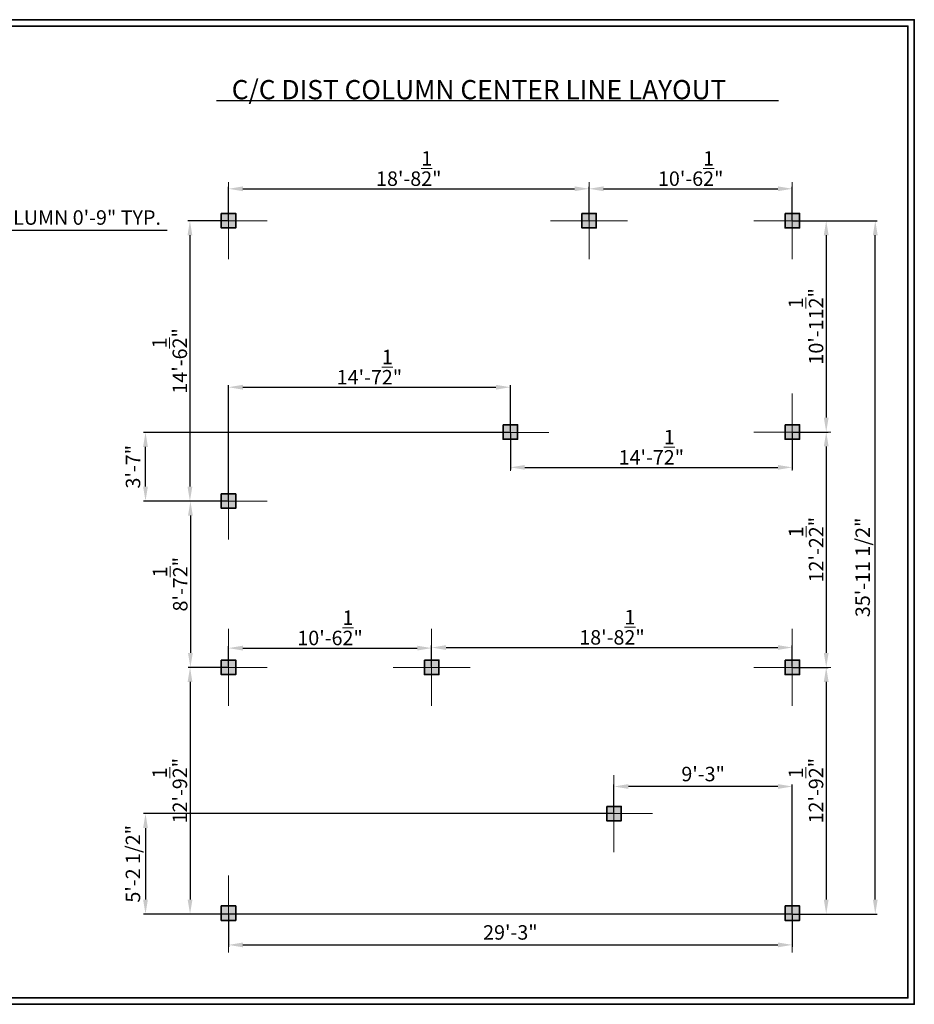
# Model space of a CAD drawing. Units: inches. Extents: x 2436 to 3928, y 1526 to 2149.
# Tile 6 of 6: x 3371 to 3928, y 1526 to 2138. Entities that reach past the tile are written whole.
import ezdxf

# ---------------------------------------------------------------- set-up
doc = ezdxf.new("R2010")
doc.units = ezdxf.units.IN
for name, color, linetype, lineweight in [('G-ANNO-TEXT', 7, 'Continuous', 25), ('G-ANNO-TTLB', 7, 'Continuous', 35), ('S-ANNO-DIMS', 2, 'Continuous', 18), ('S-COLS', 1, 'Continuous', 35), ('S-COLS-MARK', 7, 'Continuous', 13), ('S-COLS-PATT', 1, 'Continuous', 13)]:
    doc.layers.add(name, color=color, linetype=linetype, lineweight=lineweight)
doc.styles.get("Standard").update_dxf_attribs({"font": 'arial.ttf'})
doc.dimstyles.new('ISO-25', dxfattribs={"dimtxt": 9, "dimasz": 9, "dimexe": 1.25, "dimexo": 0.625, "dimgap": 2, "dimtad": 1, "dimdec": 1, "dimlunit": 4, "dimtxsty": 'Standard', "dimcen": 2.5, "dimadec": 0, "dimazin": 0, "dimtfac": 1, "dimtdec": 1, "dimtmove": 0, "dimatfit": 3, "dimfxl": 1, "dimarcsym": 0})

# ---------------------------------------------------------------- blocks, each defined once
blk = doc.blocks.new('*D10')
at = {"layer": 'Defpoints', "color": 0, "transparency": 16777216}
for p in [(3500.55, 2013.29), (3476.55, 1838.79), (3500.55, 1838.79)]:
    blk.add_point(p, dxfattribs=at)
at = {"layer": 'S-ANNO-DIMS', "color": 0, "lineweight": -2, "transparency": 16777216}
for p, q in [((3499.93, 2013.29), (3475.3, 2013.29)), ((3476.55, 2004.29), (3476.55, 1847.79)), ((3499.93, 1838.79), (3475.3, 1838.79))]:
    blk.add_line(p, q, dxfattribs=at)
at = {"layer": 'S-ANNO-DIMS', "color": 0, "transparency": 16777216}
for points in [[(3475.05, 2004.29), (3478.05, 2004.29), (3476.55, 2013.29)], [(3475.05, 1847.79), (3478.05, 1847.79), (3476.55, 1838.79)]]:
    blk.add_solid(points, dxfattribs=at)
at = {"layer": 'S-ANNO-DIMS', "color": 0, "transparency": 16777216, "insert": (3463.94, 1926.04), "char_height": 9, "attachment_point": 5, "rotation": 90}
blk.add_mtext('14\'-6{\\H1x;\\S1/2;}"', dxfattribs=at)
blk = doc.blocks.new('*D11')
at = {"layer": 'Defpoints', "color": 0, "transparency": 16777216}
for p in [(3500.55, 1838.79), (3476.86, 1735.29), (3500.55, 1735.29)]:
    blk.add_point(p, dxfattribs=at)
at = {"layer": 'S-ANNO-DIMS', "color": 0, "lineweight": -2, "transparency": 16777216}
for p, q in [((3499.93, 1838.79), (3475.61, 1838.79)), ((3476.86, 1829.79), (3476.86, 1744.29)), ((3499.93, 1735.29), (3475.61, 1735.29))]:
    blk.add_line(p, q, dxfattribs=at)
at = {"layer": 'S-ANNO-DIMS', "color": 0, "transparency": 16777216}
for points in [[(3475.36, 1829.79), (3478.36, 1829.79), (3476.86, 1838.79)], [(3475.36, 1744.29), (3478.36, 1744.29), (3476.86, 1735.29)]]:
    blk.add_solid(points, dxfattribs=at)
at = {"layer": 'S-ANNO-DIMS', "color": 0, "transparency": 16777216, "insert": (3464.24, 1787.04), "char_height": 9, "attachment_point": 5, "rotation": 90}
blk.add_mtext('8\'-7{\\H1x;\\S1/2;}"', dxfattribs=at)
blk = doc.blocks.new('*D12')
at = {"layer": 'Defpoints', "color": 0, "transparency": 16777216}
for p in [(3500.55, 1735.29), (3476.63, 1581.79), (3500.55, 1581.79)]:
    blk.add_point(p, dxfattribs=at)
at = {"layer": 'S-ANNO-DIMS', "color": 0, "lineweight": -2, "transparency": 16777216}
for p, q in [((3499.93, 1735.29), (3475.38, 1735.29)), ((3476.63, 1726.29), (3476.63, 1590.79)), ((3499.93, 1581.79), (3475.38, 1581.79))]:
    blk.add_line(p, q, dxfattribs=at)
at = {"layer": 'S-ANNO-DIMS', "color": 0, "transparency": 16777216}
for points in [[(3475.13, 1726.29), (3478.13, 1726.29), (3476.63, 1735.29)], [(3475.13, 1590.79), (3478.13, 1590.79), (3476.63, 1581.79)]]:
    blk.add_solid(points, dxfattribs=at)
at = {"layer": 'S-ANNO-DIMS', "color": 0, "transparency": 16777216, "insert": (3464.01, 1658.54), "char_height": 9, "attachment_point": 5, "rotation": 90}
blk.add_mtext('12\'-9{\\H1x;\\S1/2;}"', dxfattribs=at)
blk = doc.blocks.new('*D13')
at = {"layer": 'Defpoints', "color": 0, "transparency": 16777216}
for p in [(3500.55, 1581.79), (3851.55, 1581.79), (3851.55, 1562.57)]:
    blk.add_point(p, dxfattribs=at)
at = {"layer": 'S-ANNO-DIMS', "color": 0, "lineweight": -2, "transparency": 16777216}
for p, q in [((3500.55, 1581.16), (3500.55, 1561.32)), ((3851.55, 1581.16), (3851.55, 1561.32)), ((3509.55, 1562.57), (3842.55, 1562.57))]:
    blk.add_line(p, q, dxfattribs=at)
at = {"layer": 'S-ANNO-DIMS', "color": 0, "transparency": 16777216}
for points in [[(3509.55, 1564.07), (3509.55, 1561.07), (3500.55, 1562.57)], [(3842.55, 1564.07), (3842.55, 1561.07), (3851.55, 1562.57)]]:
    blk.add_solid(points, dxfattribs=at)
at = {"layer": 'S-ANNO-DIMS', "color": 0, "transparency": 16777216, "insert": (3676.05, 1569.17), "char_height": 9, "attachment_point": 5}
blk.add_mtext('29\'-3"', dxfattribs=at)
blk = doc.blocks.new('*D14')
at = {"layer": 'Defpoints', "color": 0, "transparency": 16777216}
for p in [(3851.55, 1735.29), (3851.55, 1581.79), (3872.67, 1581.79)]:
    blk.add_point(p, dxfattribs=at)
at = {"layer": 'S-ANNO-DIMS', "color": 0, "lineweight": -2, "transparency": 16777216}
for p, q in [((3852.18, 1735.29), (3873.92, 1735.29)), ((3872.67, 1726.29), (3872.67, 1590.79)), ((3852.18, 1581.79), (3873.92, 1581.79))]:
    blk.add_line(p, q, dxfattribs=at)
at = {"layer": 'S-ANNO-DIMS', "color": 0, "transparency": 16777216}
for points in [[(3871.17, 1726.29), (3874.17, 1726.29), (3872.67, 1735.29)], [(3871.17, 1590.79), (3874.17, 1590.79), (3872.67, 1581.79)]]:
    blk.add_solid(points, dxfattribs=at)
at = {"layer": 'S-ANNO-DIMS', "color": 0, "transparency": 16777216, "insert": (3860.05, 1658.54), "char_height": 9, "attachment_point": 5, "rotation": 90}
blk.add_mtext('12\'-9{\\H1x;\\S1/2;}"', dxfattribs=at)
blk = doc.blocks.new('*D15')
at = {"layer": 'Defpoints', "color": 0, "transparency": 16777216}
for p in [(3851.55, 1881.79), (3851.55, 1735.29), (3872.67, 1735.29)]:
    blk.add_point(p, dxfattribs=at)
at = {"layer": 'S-ANNO-DIMS', "color": 0, "lineweight": -2, "transparency": 16777216}
for p, q in [((3852.18, 1881.79), (3873.92, 1881.79)), ((3872.67, 1872.79), (3872.67, 1744.29)), ((3852.18, 1735.29), (3873.92, 1735.29))]:
    blk.add_line(p, q, dxfattribs=at)
at = {"layer": 'S-ANNO-DIMS', "color": 0, "transparency": 16777216}
for points in [[(3871.17, 1872.79), (3874.17, 1872.79), (3872.67, 1881.79)], [(3871.17, 1744.29), (3874.17, 1744.29), (3872.67, 1735.29)]]:
    blk.add_solid(points, dxfattribs=at)
at = {"layer": 'S-ANNO-DIMS', "color": 0, "transparency": 16777216, "insert": (3860.13, 1808.54), "char_height": 9, "attachment_point": 5, "rotation": 90}
blk.add_mtext('12\'-2{\\H1x;\\S1/2;}"', dxfattribs=at)
blk = doc.blocks.new('*D16')
at = {"layer": 'Defpoints', "color": 0, "transparency": 16777216}
for p in [(3851.55, 2013.29), (3851.55, 1881.79), (3872.67, 1881.79)]:
    blk.add_point(p, dxfattribs=at)
at = {"layer": 'S-ANNO-DIMS', "color": 0, "lineweight": -2, "transparency": 16777216}
for p, q in [((3852.18, 2013.29), (3873.92, 2013.29)), ((3872.67, 2004.29), (3872.67, 1890.79)), ((3852.18, 1881.79), (3873.92, 1881.79))]:
    blk.add_line(p, q, dxfattribs=at)
at = {"layer": 'S-ANNO-DIMS', "color": 0, "transparency": 16777216}
for points in [[(3871.17, 2004.29), (3874.17, 2004.29), (3872.67, 2013.29)], [(3871.17, 1890.79), (3874.17, 1890.79), (3872.67, 1881.79)]]:
    blk.add_solid(points, dxfattribs=at)
at = {"layer": 'S-ANNO-DIMS', "color": 0, "transparency": 16777216, "insert": (3860.05, 1947.54), "char_height": 9, "attachment_point": 5, "rotation": 90}
blk.add_mtext('10\'-11{\\H1x;\\S1/2;}"', dxfattribs=at)
blk = doc.blocks.new('*D17')
at = {"layer": 'Defpoints', "color": 0, "transparency": 16777216}
for p in [(3851.55, 2033.16), (3725.05, 2013.29), (3851.55, 2013.29)]:
    blk.add_point(p, dxfattribs=at)
at = {"layer": 'S-ANNO-DIMS', "color": 0, "lineweight": -2, "transparency": 16777216}
for p, q in [((3725.05, 2013.91), (3725.05, 2034.41)), ((3734.05, 2033.16), (3842.55, 2033.16)), ((3851.55, 2013.91), (3851.55, 2034.41))]:
    blk.add_line(p, q, dxfattribs=at)
at = {"layer": 'S-ANNO-DIMS', "color": 0, "transparency": 16777216}
for points in [[(3734.05, 2034.66), (3734.05, 2031.66), (3725.05, 2033.16)], [(3842.55, 2034.66), (3842.55, 2031.66), (3851.55, 2033.16)]]:
    blk.add_solid(points, dxfattribs=at)
at = {"layer": 'S-ANNO-DIMS', "color": 0, "transparency": 16777216, "insert": (3788.3, 2045.77), "char_height": 9, "attachment_point": 5}
blk.add_mtext('10\'-6{\\H1x;\\S1/2;}"', dxfattribs=at)
blk = doc.blocks.new('*D18')
at = {"layer": 'Defpoints', "color": 0, "transparency": 16777216}
for p in [(3725.05, 2033.16), (3500.55, 2013.29), (3725.05, 2013.29)]:
    blk.add_point(p, dxfattribs=at)
at = {"layer": 'S-ANNO-DIMS', "color": 0, "lineweight": -2, "transparency": 16777216}
for p, q in [((3500.55, 2013.91), (3500.55, 2034.41)), ((3509.55, 2033.16), (3716.05, 2033.16)), ((3725.05, 2013.91), (3725.05, 2034.41))]:
    blk.add_line(p, q, dxfattribs=at)
at = {"layer": 'S-ANNO-DIMS', "color": 0, "transparency": 16777216}
for points in [[(3509.55, 2034.66), (3509.55, 2031.66), (3500.55, 2033.16)], [(3716.05, 2034.66), (3716.05, 2031.66), (3725.05, 2033.16)]]:
    blk.add_solid(points, dxfattribs=at)
at = {"layer": 'S-ANNO-DIMS', "color": 0, "transparency": 16777216, "insert": (3612.8, 2045.77), "char_height": 9, "attachment_point": 5}
blk.add_mtext('18\'-8{\\H1x;\\S1/2;}"', dxfattribs=at)
blk = doc.blocks.new('*D19')
at = {"layer": 'Defpoints', "color": 0, "transparency": 16777216}
for p in [(3627.05, 1747.29), (3500.55, 1735.29), (3627.05, 1735.29)]:
    blk.add_point(p, dxfattribs=at)
at = {"layer": 'S-ANNO-DIMS', "color": 0, "lineweight": -2, "transparency": 16777216}
for p, q in [((3500.55, 1735.91), (3500.55, 1748.54)), ((3509.55, 1747.29), (3618.05, 1747.29)), ((3627.05, 1735.91), (3627.05, 1748.54))]:
    blk.add_line(p, q, dxfattribs=at)
at = {"layer": 'S-ANNO-DIMS', "color": 0, "transparency": 16777216}
for points in [[(3509.55, 1748.79), (3509.55, 1745.79), (3500.55, 1747.29)], [(3618.05, 1748.79), (3618.05, 1745.79), (3627.05, 1747.29)]]:
    blk.add_solid(points, dxfattribs=at)
at = {"layer": 'S-ANNO-DIMS', "color": 0, "transparency": 16777216, "insert": (3563.8, 1759.9), "char_height": 9, "attachment_point": 5}
blk.add_mtext('10\'-6{\\H1x;\\S1/2;}"', dxfattribs=at)
blk = doc.blocks.new('*D20')
at = {"layer": 'Defpoints', "color": 0, "transparency": 16777216}
for p in [(3851.55, 1747.65), (3627.05, 1735.29), (3851.55, 1735.29)]:
    blk.add_point(p, dxfattribs=at)
at = {"layer": 'S-ANNO-DIMS', "color": 0, "lineweight": -2, "transparency": 16777216}
for p, q in [((3627.05, 1735.91), (3627.05, 1748.9)), ((3636.05, 1747.65), (3842.55, 1747.65)), ((3851.55, 1735.91), (3851.55, 1748.9))]:
    blk.add_line(p, q, dxfattribs=at)
at = {"layer": 'S-ANNO-DIMS', "color": 0, "transparency": 16777216}
for points in [[(3636.05, 1749.15), (3636.05, 1746.15), (3627.05, 1747.65)], [(3842.55, 1749.15), (3842.55, 1746.15), (3851.55, 1747.65)]]:
    blk.add_solid(points, dxfattribs=at)
at = {"layer": 'S-ANNO-DIMS', "color": 0, "transparency": 16777216, "insert": (3739.3, 1760.27), "char_height": 9, "attachment_point": 5}
blk.add_mtext('18\'-8{\\H1x;\\S1/2;}"', dxfattribs=at)
blk = doc.blocks.new('*D21')
at = {"layer": 'Defpoints', "color": 0, "transparency": 16777216}
for p in [(3676.05, 1881.55), (3851.55, 1881.79), (3851.55, 1859.78)]:
    blk.add_point(p, dxfattribs=at)
at = {"layer": 'S-ANNO-DIMS', "color": 0, "lineweight": -2, "transparency": 16777216}
for p, q in [((3676.05, 1880.93), (3676.05, 1858.53)), ((3851.55, 1881.16), (3851.55, 1858.53)), ((3685.05, 1859.78), (3842.55, 1859.78))]:
    blk.add_line(p, q, dxfattribs=at)
at = {"layer": 'S-ANNO-DIMS', "color": 0, "transparency": 16777216}
for points in [[(3685.05, 1861.28), (3685.05, 1858.28), (3676.05, 1859.78)], [(3842.55, 1861.28), (3842.55, 1858.28), (3851.55, 1859.78)]]:
    blk.add_solid(points, dxfattribs=at)
at = {"layer": 'S-ANNO-DIMS', "color": 0, "transparency": 16777216, "insert": (3763.8, 1872.32), "char_height": 9, "attachment_point": 5}
blk.add_mtext('14\'-7{\\H1x;\\S1/2;}"', dxfattribs=at)
blk = doc.blocks.new('*D22')
at = {"layer": 'Defpoints', "color": 0, "transparency": 16777216}
for p in [(3676.05, 1909.66), (3676.05, 1881.55), (3500.55, 1838.79)]:
    blk.add_point(p, dxfattribs=at)
at = {"layer": 'S-ANNO-DIMS', "color": 0, "lineweight": -2, "transparency": 16777216}
for p, q in [((3500.55, 1839.41), (3500.55, 1910.91)), ((3509.55, 1909.66), (3667.05, 1909.66)), ((3676.05, 1882.18), (3676.05, 1910.91))]:
    blk.add_line(p, q, dxfattribs=at)
at = {"layer": 'S-ANNO-DIMS', "color": 0, "transparency": 16777216}
for points in [[(3509.55, 1911.16), (3509.55, 1908.16), (3500.55, 1909.66)], [(3667.05, 1911.16), (3667.05, 1908.16), (3676.05, 1909.66)]]:
    blk.add_solid(points, dxfattribs=at)
at = {"layer": 'S-ANNO-DIMS', "color": 0, "transparency": 16777216, "insert": (3588.3, 1922.19), "char_height": 9, "attachment_point": 5}
blk.add_mtext('14\'-7{\\H1x;\\S1/2;}"', dxfattribs=at)
blk = doc.blocks.new('*D23')
at = {"layer": 'Defpoints', "color": 0, "transparency": 16777216}
for p in [(3740.55, 1661.15), (3740.55, 1644.29), (3851.55, 1581.79)]:
    blk.add_point(p, dxfattribs=at)
at = {"layer": 'S-ANNO-DIMS', "color": 0, "lineweight": -2, "transparency": 16777216}
for p, q in [((3740.55, 1644.91), (3740.55, 1662.4)), ((3842.55, 1661.15), (3749.55, 1661.15)), ((3851.55, 1582.41), (3851.55, 1662.4))]:
    blk.add_line(p, q, dxfattribs=at)
at = {"layer": 'S-ANNO-DIMS', "color": 0, "transparency": 16777216}
for points in [[(3749.55, 1662.65), (3749.55, 1659.65), (3740.55, 1661.15)], [(3842.55, 1662.65), (3842.55, 1659.65), (3851.55, 1661.15)]]:
    blk.add_solid(points, dxfattribs=at)
at = {"layer": 'S-ANNO-DIMS', "color": 0, "transparency": 16777216, "insert": (3796.05, 1667.74), "char_height": 9, "attachment_point": 5}
blk.add_mtext('9\'-3"', dxfattribs=at)
blk = doc.blocks.new('COL-9x9-PLAN')
h = blk.add_hatch(color=256)
h.dxf.hatch_style = 1
h.paths.add_polyline_path([(9, 0), (9, 9), (0, 9), (0, 0)])
blk.add_lwpolyline([(0, 9), (9, 9), (9, 0), (0, 0)], close=True)
blk = doc.blocks.new('COLUMN-CENTER-MARK')
for q in [(24, 48), (0, 24), (48, 24), (24, 0)]:
    blk.add_line((24, 24), q)
blk = doc.blocks.new('*D30')
at = {"layer": 'Defpoints', "color": 0, "transparency": 16777216}
for p in [(3318.67, 2008.79), (3327.67, 2008.79), (3327.67, 2007.44)]:
    blk.add_point(p, dxfattribs=at)
at = {"layer": 'S-ANNO-DIMS', "color": 0, "lineweight": -2, "transparency": 16777216}
for p, q in [((3309.67, 2007.44), (3300.67, 2007.44)), ((3318.67, 2008.16), (3318.67, 2006.19)), ((3318.67, 2007.44), (3327.67, 2007.44)), ((3327.67, 2008.16), (3327.67, 2006.19)), ((3336.67, 2007.44), (3462.4, 2007.44))]:
    blk.add_line(p, q, dxfattribs=at)
at = {"layer": 'S-ANNO-DIMS', "color": 0, "transparency": 16777216}
for points in [[(3309.67, 2008.94), (3309.67, 2005.94), (3318.67, 2007.44)], [(3336.67, 2008.94), (3336.67, 2005.94), (3327.67, 2007.44)]]:
    blk.add_solid(points, dxfattribs=at)
at = {"layer": 'S-ANNO-DIMS', "color": 0, "transparency": 16777216, "insert": (3404.03, 2014.1), "char_height": 9, "attachment_point": 5}
blk.add_mtext('COLUMN 0\'-9" TYP.', dxfattribs=at)
blk = doc.blocks.new('*D78')
at = {"layer": 'Defpoints', "color": 0, "transparency": 16777216}
for p in [(3851.55, 2013.29), (3903.2, 2013.29), (3851.55, 1581.79)]:
    blk.add_point(p, dxfattribs=at)
at = {"layer": 'S-ANNO-DIMS', "color": 0, "lineweight": -2, "transparency": 16777216}
for p, q in [((3852.18, 2013.29), (3904.45, 2013.29)), ((3903.2, 1590.79), (3903.2, 2004.29)), ((3852.18, 1581.79), (3904.45, 1581.79))]:
    blk.add_line(p, q, dxfattribs=at)
at = {"layer": 'S-ANNO-DIMS', "color": 0, "transparency": 16777216}
for points in [[(3901.7, 2004.29), (3904.7, 2004.29), (3903.2, 2013.29)], [(3901.7, 1590.79), (3904.7, 1590.79), (3903.2, 1581.79)]]:
    blk.add_solid(points, dxfattribs=at)
at = {"layer": 'S-ANNO-DIMS', "color": 0, "transparency": 16777216, "insert": (3896.55, 1797.54), "char_height": 9, "attachment_point": 5, "rotation": 90}
blk.add_mtext('35\'-11 1/2"', dxfattribs=at)
blk = doc.blocks.new('*D79')
at = {"layer": 'Defpoints', "color": 0, "transparency": 16777216}
for p in [(3740.55, 1644.29), (3448.9, 1581.79), (3851.55, 1581.79)]:
    blk.add_point(p, dxfattribs=at)
at = {"layer": 'S-ANNO-DIMS', "color": 0, "lineweight": -2, "transparency": 16777216}
for p, q in [((3739.93, 1644.29), (3447.65, 1644.29)), ((3448.9, 1635.29), (3448.9, 1590.79)), ((3850.93, 1581.79), (3447.65, 1581.79))]:
    blk.add_line(p, q, dxfattribs=at)
at = {"layer": 'S-ANNO-DIMS', "color": 0, "transparency": 16777216}
for points in [[(3447.4, 1635.29), (3450.4, 1635.29), (3448.9, 1644.29)], [(3447.4, 1590.79), (3450.4, 1590.79), (3448.9, 1581.79)]]:
    blk.add_solid(points, dxfattribs=at)
at = {"layer": 'S-ANNO-DIMS', "color": 0, "transparency": 16777216, "insert": (3442.25, 1613.04), "char_height": 9, "attachment_point": 5, "rotation": 90}
blk.add_mtext('5\'-2 1/2"', dxfattribs=at)
blk = doc.blocks.new('*D80')
at = {"layer": 'Defpoints', "color": 0, "transparency": 16777216}
for p in [(3448.9, 1881.55), (3676.05, 1881.55), (3500.55, 1838.79)]:
    blk.add_point(p, dxfattribs=at)
at = {"layer": 'S-ANNO-DIMS', "color": 0, "lineweight": -2, "transparency": 16777216}
for p, q in [((3675.43, 1881.55), (3447.65, 1881.55)), ((3448.9, 1847.79), (3448.9, 1872.55)), ((3499.93, 1838.79), (3447.65, 1838.79))]:
    blk.add_line(p, q, dxfattribs=at)
at = {"layer": 'S-ANNO-DIMS', "color": 0, "transparency": 16777216}
for points in [[(3447.4, 1872.55), (3450.4, 1872.55), (3448.9, 1881.55)], [(3447.4, 1847.79), (3450.4, 1847.79), (3448.9, 1838.79)]]:
    blk.add_solid(points, dxfattribs=at)
at = {"layer": 'S-ANNO-DIMS', "color": 0, "transparency": 16777216, "insert": (3442.3, 1860.17), "char_height": 9, "attachment_point": 5, "rotation": 90}
blk.add_mtext('3\'-7"', dxfattribs=at)

msp = doc.modelspace()

# ---------------------------------------------------------------- hatches: boundary and pattern name
at = {"layer": 'S-COLS-PATT'}
h = msp.add_hatch(color=256, dxfattribs=at)
h.dxf.hatch_style = 1
h.paths.add_polyline_path([(3856.05, 1739.79), (3847.05, 1739.79), (3847.05, 1730.79), (3856.05, 1730.79)])

# ---------------------------------------------------------------- linework, layer by layer
at = {"layer": 'G-ANNO-TEXT'}
msp.add_line((3493.16, 2088.06), (3843, 2088.06), dxfattribs=at)
at = {"layer": 'G-ANNO-TTLB'}
for points in [[(2436, 2138.4), (3927.51, 2138.4), (3927.51, 1525.6), (2436, 1525.6)], [(2440, 2134.4), (3923.51, 2134.4), (3923.51, 1529.6), (2440, 1529.6)]]:
    msp.add_lwpolyline(points, close=True, dxfattribs=at)
at = {"layer": 'S-COLS'}
for p, q in [((3723.05, 2017.79), (3727.05, 2017.79)), ((3847.05, 2017.79), (3856.05, 2017.79)), ((3856.05, 2017.79), (3856.05, 2008.79))]:
    msp.add_line(p, q, dxfattribs=at)
msp.add_lwpolyline([(3847.05, 1739.79), (3856.05, 1739.79), (3856.05, 1730.79), (3847.05, 1730.79)], close=True, dxfattribs=at)
at = {"layer": 'S-COLS-MARK'}
for p, q in [((3851.55, 2017.79), (3851.55, 2008.79)), ((3720.55, 2013.29), (3729.55, 2013.29)), ((3847.05, 2013.29), (3856.05, 2013.29)), ((3847.05, 1881.79), (3856.05, 1881.79)), ((3847.05, 1735.29), (3856.05, 1735.29))]:
    msp.add_line(p, q, dxfattribs=at)

# ---------------------------------------------------------------- block references
at = {"layer": 'S-COLS'}
for p in [(3496.05, 2008.79), (3720.55, 2008.79), (3847.05, 2008.79), (3671.55, 1877.29), (3847.05, 1877.29), (3496.05, 1834.29), (3496.05, 1730.79), (3622.55, 1730.79), (3736.05, 1639.79), (3496.05, 1577.79), (3847.05, 1577.79)]:
    msp.add_blockref('COL-9x9-PLAN', p, dxfattribs=at)
at = {"layer": 'S-COLS-MARK'}
for p, rotation in [((3476.55, 2037.29), 270.0000000000011), ((3701.05, 2037.29), 270.0000000000005), ((3827.55, 2037.29), 270.0000000000011), ((3827.55, 1905.79), 270.0000000000017), ((3476.55, 1862.79), 270.0000000000011), ((3476.55, 1759.29), 270.0000000000017), ((3603.05, 1759.29), 270.0000000000017), ((3827.55, 1759.29), 270.0000000000017), ((3716.55, 1668.29), 270.0000000000005), ((3476.55, 1605.79), 270.0000000000011), ((3827.55, 1605.79), 270.0000000000017)]:
    msp.add_blockref('COLUMN-CENTER-MARK', p, dxfattribs=dict(at, rotation=rotation))
msp.add_blockref('COLUMN-CENTER-MARK', (3652.05, 1857.55), dxfattribs=at)

# ---------------------------------------------------------------- texts
at = {"layer": 'G-ANNO-TEXT'}
msp.add_text('C/C DIST COLUMN CENTER LINE LAYOUT', height=12, dxfattribs=at).set_placement((3502.57, 2088.86))

# ---------------------------------------------------------------- dimensions: what is measured, and where the dimension line sits
at = {"layer": 'S-ANNO-DIMS'}
for base, p1, p2, picture, middle in [((3725.05, 2033.16), (3500.55, 2013.29), (3725.05, 2013.29), '*D18', (3612.8, 2045.77)), ((3851.55, 2033.16), (3725.05, 2013.29), (3851.55, 2013.29), '*D17', (3788.3, 2045.77)), ((3676.05, 1909.66), (3500.55, 1838.79), (3676.05, 1881.55), '*D22', (3588.3, 1922.19)), ((3851.55, 1859.78), (3676.05, 1881.55), (3851.55, 1881.79), '*D21', (3763.8, 1872.32)), ((3851.55, 1747.65), (3627.05, 1735.29), (3851.55, 1735.29), '*D20', (3739.3, 1760.27)), ((3627.05, 1747.29), (3500.55, 1735.29), (3627.05, 1735.29), '*D19', (3563.8, 1759.9)), ((3740.55, 1661.15), (3851.55, 1581.79), (3740.55, 1644.29), '*D23', (3796.05, 1667.74)), ((3851.55, 1562.57), (3500.55, 1581.79), (3851.55, 1581.79), '*D13', (3676.05, 1569.17))]:
    dim = msp.add_linear_dim(base=base, p1=p1, p2=p2, dimstyle='ISO-25', override={"dimclrd": 0, "dimclre": 0, "dimclrt": 0}, dxfattribs=at)
    dim.commit()
    dim.dimension.update_dxf_attribs({"geometry": picture, "text_midpoint": middle})
dim = msp.add_linear_dim(base=(3327.67, 2007.44), p1=(3318.67, 2008.79), p2=(3327.67, 2008.79), text='COLUMN <> TYP.', dimstyle='ISO-25', override={"dimdec": 1, "dimlfac": 1, "dimrnd": 0, "dimzin": 1, "dimdsep": 46, "dimlunit": 4, "dimfrac": 2}, dxfattribs=at)
dim.commit()
dim.dimension.update_dxf_attribs({"geometry": '*D30', "text_midpoint": (3404.03, 2014.1)})
for base, p1, p2, override, picture, middle in [((3476.55, 1838.79), (3500.55, 2013.29), (3500.55, 1838.79), {"dimclrd": 0, "dimclre": 0, "dimclrt": 0}, '*D10', (3463.94, 1926.04)), ((3872.67, 1881.79), (3851.55, 2013.29), (3851.55, 1881.79), {"dimclrd": 0, "dimclre": 0, "dimclrt": 0}, '*D16', (3860.05, 1947.54)), ((3903.2, 2013.29), (3851.55, 1581.79), (3851.55, 2013.29), {"dimdec": 1, "dimlfac": 1, "dimrnd": 0, "dimzin": 1, "dimdsep": 46, "dimlunit": 4, "dimfrac": 2}, '*D78', (3896.55, 1797.54)), ((3448.9, 1881.55), (3500.55, 1838.79), (3676.05, 1881.55), {"dimdec": 1, "dimlfac": 1, "dimrnd": 0, "dimzin": 1, "dimdsep": 46, "dimlunit": 4, "dimfrac": 2}, '*D80', (3442.3, 1860.17)), ((3872.67, 1735.29), (3851.55, 1881.79), (3851.55, 1735.29), {"dimclrd": 0, "dimclre": 0, "dimclrt": 0}, '*D15', (3860.13, 1808.54)), ((3476.86, 1735.29), (3500.55, 1838.79), (3500.55, 1735.29), {"dimclrd": 0, "dimclre": 0, "dimclrt": 0}, '*D11', (3464.24, 1787.04)), ((3476.63, 1581.79), (3500.55, 1735.29), (3500.55, 1581.79), {"dimclrd": 0, "dimclre": 0, "dimclrt": 0}, '*D12', (3464.01, 1658.54)), ((3872.67, 1581.79), (3851.55, 1735.29), (3851.55, 1581.79), {"dimclrd": 0, "dimclre": 0, "dimclrt": 0}, '*D14', (3860.05, 1658.54)), ((3448.9, 1581.79), (3740.55, 1644.29), (3851.55, 1581.79), {"dimdec": 1, "dimlfac": 1, "dimrnd": 0, "dimzin": 1, "dimdsep": 46, "dimlunit": 4, "dimfrac": 2}, '*D79', (3442.25, 1613.04))]:
    dim = msp.add_linear_dim(base=base, p1=p1, p2=p2, angle=90, dimstyle='ISO-25', override=override, dxfattribs=at)
    dim.commit()
    dim.dimension.update_dxf_attribs({"geometry": picture, "text_midpoint": middle})

doc.saveas('drawing.dxf')
